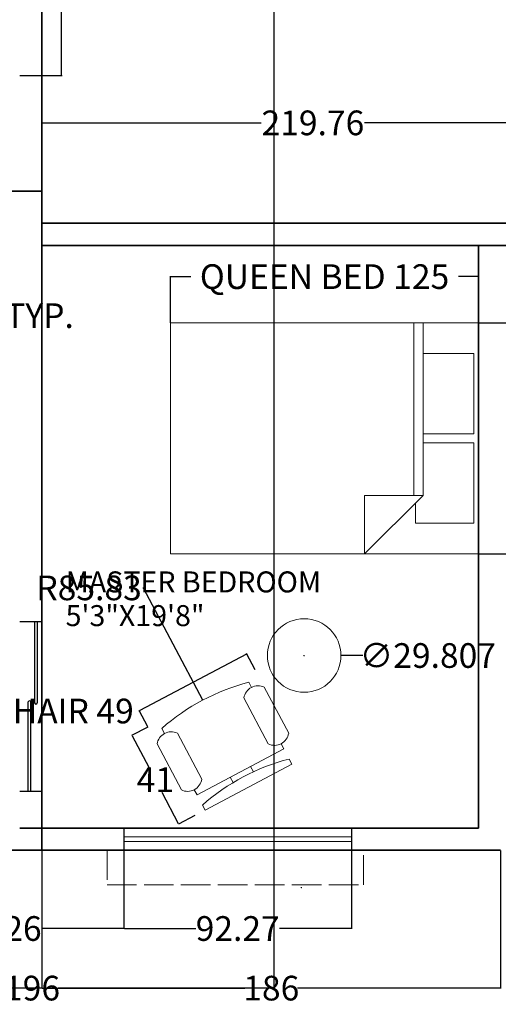
# Model space of a CAD drawing. Units: inches. Extents: x 135 to 880, y 60 to 879.
# Tile 2 of 5: x 363 to 557, y 60 to 459. Entities that reach past the tile are written whole.
import ezdxf

# ---------------------------------------------------------------- set-up
doc = ezdxf.new("R2010")
doc.units = ezdxf.units.IN
doc.header["$MEASUREMENT"] = 0
doc.linetypes.add('ACAD_ISO02W100', pattern=[15, 12, -3])
for name, color, linetype, lineweight in [('A-ANNO-DIMS', 2, 'Continuous', 18), ('A-AREA-IDEN', 7, 'Continuous', 18), ('A-DOOR', 3, 'Continuous', 25), ('A-FURN', 8, 'Continuous', 18), ('A-GLAZ', 4, 'Continuous', 18), ('A-ROOF-OVHD', 8, 'ACAD_ISO02W100', 18), ('A-WALL', 7, 'Continuous', 35)]:
    doc.layers.add(name, color=color, linetype=linetype, lineweight=lineweight)
doc.styles.get("Standard").update_dxf_attribs({"font": 'arial.ttf'})
doc.dimstyles.get("Standard").update_dxf_attribs({"dimtxt": 10, "dimasz": 0.18, "dimexe": 0.18, "dimexo": 0.0625, "dimgap": 0.09, "dimtad": 0, "dimtih": 1, "dimtoh": 1, "dimdec": 0, "dimzin": 0, "dimdsep": 46, "dimlunit": 3, "dimtxsty": 'Standard', "dimcen": 0.09, "dimadec": 0, "dimazin": 0, "dimtfac": 1, "dimtdec": 0, "dimtofl": 0, "dimtmove": 0, "dimatfit": 3, "dimfxl": 1, "dimtolj": 1, "dimtzin": 0, "dimarcsym": 0})

# ---------------------------------------------------------------- blocks, each defined once
blk = doc.blocks.new('Chair - Desk')
for p, q in [((-8.5, 0), (-8.5, -1)), ((-8.5, 0), (8.5, 0)), ((8.5, 0), (8.5, -1)), ((-8.5, -3), (-8.5, -4)), ((-8.5, -3), (8.5, -3)), ((-2, -3), (-2, -1.9355)), ((2, -1.9576), (2, -3)), ((8.5, -3), (8.5, -4)), ((-10.5, -5), (-10.5, -14)), ((-6.5, -14), (-6.5, -5)), ((6.5, -5), (6.5, -14)), ((10.5, -14), (10.5, -5)), ((-8.5, -15), (-8.5, -16)), ((8.5, -15), (8.5, -16))]:
    blk.add_line(p, q)
for centre, radius, start, end in [((0, 34.625), 36.625, 256.5803, 283.4197), ((-8.5, -6.5), 2.5, 36.8699, 143.1301), ((8.5, -6.5), 2.5, 36.8699, 143.1301), ((-8.5, -12.5), 2.5, 216.8699, 323.1301), ((8.5, -12.5), 2.5, 216.8699, 323.1301), ((0, 19.625), 36.625, 256.5803, 283.4197)]:
    blk.add_arc(centre, radius, start, end)
blk = doc.blocks.new('Bed - Queen')
for p, q in [((0, -80.00003), (0, 0)), ((0, 0), (59.99999, 0)), ((59.99999, 0), (59.99999, -80.00003)), ((7.99999, -1.2), (28.79998, -1.2)), ((7.99999, -14.4), (7.99999, -1.2)), ((28.79998, -1.2), (28.79998, -14.4)), ((31.19999, -1.2), (51.99999, -1.2)), ((31.19999, -14.4), (31.19999, -1.2)), ((51.99999, -1.2), (51.99999, -16.4)), ((0, -14.4), (44.8, -14.4)), ((59.99999, -29.6), (44.8, -14.4)), ((44.8, -14.4), (44.8, -29.6)), ((44.8, -16.8), (0, -16.8)), ((51.99999, -16.4), (46.79936, -16.4)), ((44.8, -29.6), (59.99999, -29.6)), ((59.99999, -80.00003), (0, -80.00003))]:
    blk.add_line(p, q)
blk = doc.blocks.new('*D14')
at = {"layer": 'A-ANNO-DIMS', "color": 0, "lineweight": -2, "transparency": 16777216}
for p, q in [((454.9, 202.13), (411.72, 179.27)), ((458.48, 195.75), (454.97, 202.38)), ((411.4, 179.11), (411.22, 179.11)), ((411.56, 179.19), (411.4, 179.11)), ((414.99, 172.72), (411.48, 179.35))]:
    blk.add_line(p, q, dxfattribs=at)
at = {"layer": 'A-ANNO-DIMS', "color": 0, "transparency": 16777216}
for points in [[(454.88, 202.16), (454.91, 202.11), (455.05, 202.22)], [(411.71, 179.3), (411.73, 179.25), (411.56, 179.19)]]:
    blk.add_solid(points, dxfattribs=at)
at = {"layer": 'Defpoints', "color": 0, "transparency": 16777216}
for p in [(458.51, 195.69), (411.56, 179.19), (415.01, 172.67)]:
    blk.add_point(p, dxfattribs=at)
at = {"layer": 'A-ANNO-DIMS', "color": 0, "transparency": 16777216, "insert": (380.34, 179.11), "char_height": 10, "attachment_point": 5}
blk.add_mtext('\\A1;CHAIR 49', dxfattribs=at)
blk = doc.blocks.new('*D15')
at = {"layer": 'A-ANNO-DIMS', "color": 0, "lineweight": -2, "transparency": 16777216}
for p, q in [((414.96, 172.64), (408.33, 169.13)), ((408.57, 169.05), (415.29, 156.37)), ((427.41, 133.47), (420.7, 146.15)), ((433.97, 136.74), (427.34, 133.23))]:
    blk.add_line(p, q, dxfattribs=at)
at = {"layer": 'A-ANNO-DIMS', "color": 0, "transparency": 16777216}
for points in [[(408.6, 169.07), (408.55, 169.04), (408.49, 169.21)], [(427.44, 133.48), (427.39, 133.46), (427.5, 133.31)]]:
    blk.add_solid(points, dxfattribs=at)
at = {"layer": 'Defpoints', "color": 0, "transparency": 16777216}
for p in [(415.01, 172.67), (434.02, 136.76), (427.5, 133.31)]:
    blk.add_point(p, dxfattribs=at)
at = {"layer": 'A-ANNO-DIMS', "color": 0, "transparency": 16777216, "insert": (417.99, 151.26), "char_height": 10, "attachment_point": 5}
blk.add_mtext('\\A1;41', dxfattribs=at)
blk = doc.blocks.new('*D25')
at = {"layer": 'A-ANNO-DIMS', "color": 0, "lineweight": -2, "transparency": 16777216}
for p, q in [((363.04, 521.66), (380.17, 521.66)), ((379.99, 521.48), (379.99, 484.31)), ((379.99, 436.75), (379.99, 473.92)), ((363.04, 436.57), (380.17, 436.57))]:
    blk.add_line(p, q, dxfattribs=at)
at = {"layer": 'A-ANNO-DIMS', "color": 0, "transparency": 16777216}
for points in [[(379.96, 521.48), (380.02, 521.48), (379.99, 521.66)], [(379.96, 436.75), (380.02, 436.75), (379.99, 436.57)]]:
    blk.add_solid(points, dxfattribs=at)
at = {"layer": 'Defpoints', "color": 0, "transparency": 16777216}
for p in [(362.98, 521.66), (362.98, 436.57), (379.99, 436.57)]:
    blk.add_point(p, dxfattribs=at)
at = {"layer": 'A-ANNO-DIMS', "color": 0, "transparency": 16777216, "insert": (379.99, 479.12), "char_height": 10, "attachment_point": 5}
blk.add_mtext('\\A1;85', dxfattribs=at)
blk = doc.blocks.new('*D26')
at = {"layer": 'A-ANNO-DIMS', "color": 0, "lineweight": -2, "transparency": 16777216}
for p, q in [((424.17, 336.45), (424.17, 355.29)), ((424.35, 355.11), (432.33, 355.11)), ((548.8, 355.11), (540.82, 355.11)), ((548.98, 336.45), (548.98, 355.29))]:
    blk.add_line(p, q, dxfattribs=at)
at = {"layer": 'A-ANNO-DIMS', "color": 0, "transparency": 16777216}
for points in [[(424.35, 355.14), (424.35, 355.08), (424.17, 355.11)], [(548.8, 355.14), (548.8, 355.08), (548.98, 355.11)]]:
    blk.add_solid(points, dxfattribs=at)
at = {"layer": 'Defpoints', "color": 0, "transparency": 16777216}
for p in [(548.98, 355.11), (424.17, 336.39), (548.98, 336.39)]:
    blk.add_point(p, dxfattribs=at)
at = {"layer": 'A-ANNO-DIMS', "color": 0, "transparency": 16777216, "insert": (486.57, 355.11), "char_height": 10, "attachment_point": 5}
blk.add_mtext('\\A1;QUEEN BED 125', dxfattribs=at)
blk = doc.blocks.new('*D27')
at = {"layer": 'A-ANNO-DIMS', "color": 0, "lineweight": -2, "transparency": 16777216}
for p, q in [((549.04, 336.39), (567.88, 336.39)), ((567.7, 336.21), (567.7, 294.78)), ((567.7, 242.96), (567.7, 284.39)), ((549.04, 242.78), (567.88, 242.78))]:
    blk.add_line(p, q, dxfattribs=at)
at = {"layer": 'A-ANNO-DIMS', "color": 0, "transparency": 16777216}
for points in [[(567.67, 336.21), (567.73, 336.21), (567.7, 336.39)], [(567.67, 242.96), (567.73, 242.96), (567.7, 242.78)]]:
    blk.add_solid(points, dxfattribs=at)
at = {"layer": 'Defpoints', "color": 0, "transparency": 16777216}
for p in [(548.98, 336.39), (548.98, 242.78), (567.7, 242.78)]:
    blk.add_point(p, dxfattribs=at)
at = {"layer": 'A-ANNO-DIMS', "color": 0, "transparency": 16777216, "insert": (567.7, 289.58), "char_height": 10, "attachment_point": 5}
blk.add_mtext('\\A1;94', dxfattribs=at)
blk = doc.blocks.new('*D32')
at = {"layer": 'A-ANNO-DIMS', "color": 0, "lineweight": -2, "transparency": 16777216}
for p, q in [((257.98, 344.64), (257.98, 339.12)), ((293.98, 344.64), (293.98, 339.12)), ((258.16, 339.3), (293.8, 339.3)), ((293.98, 339.3), (294.16, 339.3))]:
    blk.add_line(p, q, dxfattribs=at)
at = {"layer": 'A-ANNO-DIMS', "color": 0, "transparency": 16777216}
for points in [[(258.16, 339.33), (258.16, 339.27), (257.98, 339.3)], [(293.8, 339.33), (293.8, 339.27), (293.98, 339.3)]]:
    blk.add_solid(points, dxfattribs=at)
at = {"layer": 'Defpoints', "color": 0, "transparency": 16777216}
for p in [(257.98, 344.7), (293.98, 344.7), (293.98, 339.3)]:
    blk.add_point(p, dxfattribs=at)
at = {"layer": 'A-ANNO-DIMS', "color": 0, "transparency": 16777216, "insert": (341.23, 339.3), "char_height": 10, "attachment_point": 5}
blk.add_mtext('\\A1;DOOR 36 TYP.', dxfattribs=at)
blk = doc.blocks.new('*D54')
at = {"layer": 'A-ANNO-DIMS', "color": 0, "lineweight": -2, "transparency": 16777216}
for p, q in [((192.98, 122.64), (192.98, 66.67)), ((371.98, 122.64), (371.98, 66.67)), ((193.16, 66.85), (271.8, 66.85)), ((371.8, 66.85), (293.15, 66.85))]:
    blk.add_line(p, q, dxfattribs=at)
at = {"layer": 'A-ANNO-DIMS', "color": 0, "transparency": 16777216}
for points in [[(193.16, 66.88), (193.16, 66.82), (192.98, 66.85)], [(371.8, 66.88), (371.8, 66.82), (371.98, 66.85)]]:
    blk.add_solid(points, dxfattribs=at)
at = {"layer": 'Defpoints', "color": 0, "transparency": 16777216}
for p in [(192.98, 122.7), (371.98, 122.7), (371.98, 66.85)]:
    blk.add_point(p, dxfattribs=at)
at = {"layer": 'A-ANNO-DIMS', "color": 0, "transparency": 16777216, "insert": (282.48, 66.85), "char_height": 10, "attachment_point": 5}
blk.add_mtext('\\A1;179', dxfattribs=at)
blk = doc.blocks.new('*D55')
at = {"layer": 'A-ANNO-DIMS', "color": 0, "lineweight": -2, "transparency": 16777216}
for p, q in [((371.98, 122.64), (371.98, 66.67)), ((557.98, 122.64), (557.98, 66.67)), ((372.16, 66.85), (454.31, 66.85)), ((557.8, 66.85), (475.64, 66.85))]:
    blk.add_line(p, q, dxfattribs=at)
at = {"layer": 'A-ANNO-DIMS', "color": 0, "transparency": 16777216}
for points in [[(372.16, 66.88), (372.16, 66.82), (371.98, 66.85)], [(557.8, 66.88), (557.8, 66.82), (557.98, 66.85)]]:
    blk.add_solid(points, dxfattribs=at)
at = {"layer": 'Defpoints', "color": 0, "transparency": 16777216}
for p in [(371.98, 122.7), (557.98, 122.7), (557.98, 66.85)]:
    blk.add_point(p, dxfattribs=at)
at = {"layer": 'A-ANNO-DIMS', "color": 0, "transparency": 16777216, "insert": (464.98, 66.85), "char_height": 10, "attachment_point": 5}
blk.add_mtext('\\A1;186', dxfattribs=at)
blk = doc.blocks.new('*D59')
at = {"layer": 'A-ANNO-DIMS', "color": 0, "lineweight": -2, "transparency": 16777216}
for p, q in [((371.98, 131.64), (371.98, 90.82)), ((405.23, 131.64), (405.23, 90.82)), ((371.98, 91), (371.8, 91)), ((405.05, 91), (372.16, 91))]:
    blk.add_line(p, q, dxfattribs=at)
at = {"layer": 'A-ANNO-DIMS', "color": 0, "transparency": 16777216}
for points in [[(372.16, 91.03), (372.16, 90.97), (371.98, 91)], [(405.05, 91.03), (405.05, 90.97), (405.23, 91)]]:
    blk.add_solid(points, dxfattribs=at)
at = {"layer": 'Defpoints', "color": 0, "transparency": 16777216}
for p in [(371.98, 131.7), (405.23, 131.7), (371.98, 91)]:
    blk.add_point(p, dxfattribs=at)
at = {"layer": 'A-ANNO-DIMS', "color": 0, "transparency": 16777216, "insert": (354.84, 91), "char_height": 10, "attachment_point": 5}
blk.add_mtext('\\A1;33.26', dxfattribs=at)
blk = doc.blocks.new('*D60')
at = {"layer": 'A-ANNO-DIMS', "color": 0, "lineweight": -2, "transparency": 16777216}
for p, q in [((405.23, 131.64), (405.23, 90.82)), ((497.5, 131.64), (497.5, 90.82)), ((405.41, 91), (434.4, 91)), ((497.32, 91), (468.33, 91))]:
    blk.add_line(p, q, dxfattribs=at)
at = {"layer": 'A-ANNO-DIMS', "color": 0, "transparency": 16777216}
for points in [[(405.41, 91.03), (405.41, 90.97), (405.23, 91)], [(497.32, 91.03), (497.32, 90.97), (497.5, 91)]]:
    blk.add_solid(points, dxfattribs=at)
at = {"layer": 'Defpoints', "color": 0, "transparency": 16777216}
for p in [(405.23, 131.7), (497.5, 131.7), (405.23, 91)]:
    blk.add_point(p, dxfattribs=at)
at = {"layer": 'A-ANNO-DIMS', "color": 0, "transparency": 16777216, "insert": (451.37, 91), "char_height": 10, "attachment_point": 5}
blk.add_mtext('\\A1;92.27', dxfattribs=at)
blk = doc.blocks.new('*D72')
at = {"layer": 'A-ANNO-DIMS', "color": 0, "lineweight": -2, "transparency": 16777216}
for p, q in [((269.98, 822.64), (269.98, 66.67)), ((465.98, 822.64), (465.98, 66.67)), ((270.16, 66.85), (357.31, 66.85)), ((465.8, 66.85), (378.64, 66.85))]:
    blk.add_line(p, q, dxfattribs=at)
at = {"layer": 'A-ANNO-DIMS', "color": 0, "transparency": 16777216}
for points in [[(270.16, 66.88), (270.16, 66.82), (269.98, 66.85)], [(465.8, 66.88), (465.8, 66.82), (465.98, 66.85)]]:
    blk.add_solid(points, dxfattribs=at)
at = {"layer": 'Defpoints', "color": 0, "transparency": 16777216}
for p in [(269.98, 822.7), (465.98, 822.7), (465.98, 66.85)]:
    blk.add_point(p, dxfattribs=at)
at = {"layer": 'A-ANNO-DIMS', "color": 0, "transparency": 16777216, "insert": (367.98, 66.85), "char_height": 10, "attachment_point": 5}
blk.add_mtext('\\A1;196', dxfattribs=at)
blk = doc.blocks.new('*D74')
at = {"layer": 'A-ANNO-DIMS', "color": 0, "lineweight": -2, "transparency": 16777216}
for p, q in [((371.98, 376.76), (371.98, 417.58)), ((372.16, 417.4), (460.93, 417.4)), ((591.56, 417.4), (502.79, 417.4)), ((591.74, 376.76), (591.74, 417.58))]:
    blk.add_line(p, q, dxfattribs=at)
at = {"layer": 'A-ANNO-DIMS', "color": 0, "transparency": 16777216}
for points in [[(372.16, 417.43), (372.16, 417.37), (371.98, 417.4)], [(591.56, 417.43), (591.56, 417.37), (591.74, 417.4)]]:
    blk.add_solid(points, dxfattribs=at)
at = {"layer": 'Defpoints', "color": 0, "transparency": 16777216}
for p in [(591.74, 417.4), (371.98, 376.7), (591.74, 376.7)]:
    blk.add_point(p, dxfattribs=at)
at = {"layer": 'A-ANNO-DIMS', "color": 0, "transparency": 16777216, "insert": (481.86, 417.4), "char_height": 10, "attachment_point": 5}
blk.add_mtext('\\A1;219.76', dxfattribs=at)
blk = doc.blocks.new('*D80')
at = {"layer": 'A-ANNO-DIMS', "color": 0, "lineweight": -2, "transparency": 16777216}
for p, q in [((478.22, 201.6), (478.4, 201.6)), ((478.31, 201.51), (478.31, 201.69)), ((502.15, 201.6), (493.39, 201.6))]:
    blk.add_line(p, q, dxfattribs=at)
at = {"layer": 'A-ANNO-DIMS', "color": 0, "transparency": 16777216}
blk.add_solid([(493.39, 201.63), (493.39, 201.57), (493.21, 201.6)], dxfattribs=at)
at = {"layer": 'Defpoints', "color": 0, "transparency": 16777216}
for p in [(463.4, 201.6), (493.21, 201.6)]:
    blk.add_point(p, dxfattribs=at)
at = {"layer": 'A-ANNO-DIMS', "color": 0, "transparency": 16777216, "insert": (528.44, 201.6), "char_height": 10, "attachment_point": 5}
blk.add_mtext('\\A1;∅29.807', dxfattribs=at)
blk = doc.blocks.new('*D85')
at = {"layer": 'A-ANNO-DIMS', "color": 0, "lineweight": -2, "transparency": 16777216}
for p, q in [((412.85, 229), (413.03, 229)), ((413.03, 229), (437.04, 183.65)), ((477.29, 107.54), (477.29, 107.72)), ((477.2, 107.63), (477.38, 107.63))]:
    blk.add_line(p, q, dxfattribs=at)
at = {"layer": 'A-ANNO-DIMS', "color": 0, "transparency": 16777216}
blk.add_solid([(437.07, 183.66), (437.02, 183.63), (437.13, 183.49)], dxfattribs=at)
at = {"layer": 'Defpoints', "color": 0, "transparency": 16777216}
for p in [(437.13, 183.49), (477.29, 107.63)]:
    blk.add_point(p, dxfattribs=at)
at = {"layer": 'A-ANNO-DIMS', "color": 0, "transparency": 16777216, "insert": (391.1, 229), "char_height": 10, "attachment_point": 5}
blk.add_mtext('\\A1;R85.83', dxfattribs=at)

msp = doc.modelspace()

# ---------------------------------------------------------------- linework, layer by layer
at = {"layer": 'A-DOOR'}
for p, q in [((362.9753, 215.4206), (371.9753, 215.4206)), ((369.0511, 215.4206), (369.0511, 182.3912)), ((370.0511, 215.4206), (370.0511, 182.3912)), ((366.4743, 146.6389), (366.4743, 182.8082)), ((367.4743, 146.6389), (367.4743, 182.8082)), ((362.9753, 146.6389), (371.9753, 146.6389))]:
    msp.add_line(p, q, dxfattribs=at)
for centre, start, end in [((366.9743, 182.8082), 0, 180), ((369.5511, 182.3912), 180, 0)]:
    msp.add_arc(centre, 0.5, start, end, dxfattribs=at)
at = {"layer": 'A-FURN'}
msp.add_circle((478.3065, 201.5966), 14.9034, dxfattribs=at)
at = {"layer": 'A-GLAZ'}
for p, q in [((405.2334, 131.7014), (405.2334, 122.7014)), ((497.5015, 131.7014), (497.5015, 131.7014)), ((497.5015, 131.7014), (497.5015, 122.7014)), ((405.2334, 128.2014), (497.5015, 128.2014)), ((405.2334, 126.2014), (497.5015, 126.2014))]:
    msp.add_line(p, q, dxfattribs=at)
at = {"layer": 'A-ROOF-OVHD'}
for p, q in [((398.3792, 122.7014), (398.3792, 108.694)), ((502.332, 108.694), (502.332, 122.7014)), ((398.3792, 108.694), (502.332, 108.694))]:
    msp.add_line(p, q, dxfattribs=at)
at = {"layer": 'A-WALL'}
for p, q in [((371.9753, 559.7014), (371.9753, 389.7014)), ((371.9753, 389.7014), (343.1077, 389.7014)), ((371.9753, 258.7014), (371.9753, 389.7014)), ((775.9753, 376.7014), (371.9753, 376.7014)), ((784.9753, 367.7014), (371.9753, 367.7014)), ((548.9753, 131.7014), (548.9753, 367.7014)), ((548.9753, 367.7014), (557.9753, 367.7014)), ((371.9753, 122.7014), (371.9753, 258.7014)), ((362.9753, 131.7014), (371.9753, 131.7014)), ((371.9753, 131.7014), (548.9753, 131.7014)), ((192.9753, 122.7014), (371.9753, 122.7014)), ((371.9753, 122.7014), (557.9753, 122.7014))]:
    msp.add_line(p, q, dxfattribs=at)

# ---------------------------------------------------------------- block references
at = {"layer": 'A-FURN'}
for name, p, xscale, yscale, zscale, rotation in [('Bed - Queen', (548.9753, 336.3855), 1.560037282092657, 1.560037282092657, 1.560037282092657, 270), ('Chair - Desk', (455.7677, 148.2781), 2.343520009776944, 2.343520009776944, 2.343520009776944, 207.8972710309477)]:
    msp.add_blockref(name, p, dxfattribs=dict(at, xscale=xscale, yscale=yscale, zscale=zscale, rotation=rotation))

# ---------------------------------------------------------------- texts
at = {"layer": 'A-AREA-IDEN'}
for s, height, p in [('MASTER BEDROOM ', 8.505802, (381.5975, 227.1713)), ('5\'3"X19\'8"', 8.5058, (381.5975, 213.5075))]:
    msp.add_text(s, height=height, dxfattribs=at).set_placement(p)

# ---------------------------------------------------------------- dimensions: what is measured, and where the dimension line sits
at = {"layer": 'A-ANNO-DIMS'}
for base, p1, p2, override, picture, middle in [((465.9753, 66.853), (269.9753, 822.7014), (465.9753, 822.7014), {"dimdec": 0, "dimlfac": 1, "dimrnd": 0, "dimzin": 0, "dimdsep": 46, "dimlunit": 2}, '*D72', (367.9753, 66.853)), ((591.7388, 417.4014), (371.9753, 376.7014), (591.7388, 376.7014), {"dimdec": 2, "dimlfac": 1, "dimrnd": 0, "dimzin": 0, "dimdsep": 46, "dimlunit": 2}, '*D74', (481.8571, 417.4014)), ((371.9753, 66.853), (192.9753, 122.7014), (371.9753, 122.7014), {"dimdec": 0, "dimlfac": 1, "dimrnd": 0, "dimzin": 0, "dimdsep": 46, "dimlunit": 2}, '*D54', (282.4753, 66.853)), ((557.9753, 66.853), (371.9753, 122.7014), (557.9753, 122.7014), {"dimdec": 0, "dimlfac": 1, "dimrnd": 0, "dimzin": 0, "dimdsep": 46, "dimlunit": 2}, '*D55', (464.9753, 66.853))]:
    dim = msp.add_linear_dim(base=base, p1=p1, p2=p2, dimstyle='Standard', override=override, dxfattribs=at)
    dim.commit()
    dim.dimension.update_dxf_attribs({"geometry": picture, "text_midpoint": middle})
for base, p1, p2, angle, override, picture, middle in [((379.993, 436.5713), (362.9753, 521.6594), (362.9753, 436.5713), 270, {"dimdec": 0, "dimlfac": 1, "dimrnd": 0, "dimzin": 0, "dimdsep": 46, "dimlunit": 2}, '*D25', (379.993, 479.1154)), ((567.6958, 242.7833), (548.9753, 336.3855), (548.9753, 242.7833), 270, {"dimdec": 0, "dimlfac": 1, "dimrnd": 0, "dimzin": 0, "dimdsep": 46, "dimlunit": 2}, '*D27', (567.6958, 289.5844)), ((427.4961, 133.3108), (415.0143, 172.6652), (434.0203, 136.7648), 297.897271, {"dimdec": 0, "dimlfac": 1, "dimrnd": 0, "dimzin": 0, "dimdsep": 46, "dimlunit": 2}, '*D15', (417.9931, 151.261)), ((371.9753, 91.0014), (405.2334, 131.7014), (371.9753, 131.7014), 180, {"dimdec": 2, "dimlfac": 1, "dimrnd": 0, "dimzin": 0, "dimdsep": 46, "dimlunit": 2}, '*D59', (354.8397, 91.0014)), ((405.2334, 91.0014), (497.5015, 131.7014), (405.2334, 131.7014), 180, {"dimdec": 2, "dimlfac": 1, "dimrnd": 0, "dimzin": 0, "dimdsep": 46, "dimlunit": 2}, '*D60', (451.3674, 91.0014))]:
    dim = msp.add_linear_dim(base=base, p1=p1, p2=p2, angle=angle, dimstyle='Standard', override=override, dxfattribs=at)
    dim.commit()
    dim.dimension.update_dxf_attribs({"geometry": picture, "text_midpoint": middle})
for base, p1, p2, text, picture, middle in [((548.9753, 355.106), (424.1723, 336.3855), (548.9753, 336.3855), 'QUEEN BED <>', '*D26', (486.5738, 355.106)), ((293.9753, 339.3014), (257.9753, 344.7014), (293.9753, 344.7014), 'DOOR <> TYP.', '*D32', (341.2303, 339.3014))]:
    dim = msp.add_linear_dim(base=base, p1=p1, p2=p2, text=text, dimstyle='Standard', override={"dimdec": 0, "dimlfac": 1, "dimrnd": 0, "dimzin": 0, "dimdsep": 46, "dimlunit": 2}, dxfattribs=at)
    dim.commit()
    dim.dimension.update_dxf_attribs({"geometry": picture, "text_midpoint": middle})
dim = msp.add_radius_dim(center=(477.2866, 107.6313), mpoint=(437.127, 183.488), dimstyle='Standard', override={"dimdec": 2, "dimlfac": 1, "dimrnd": 0, "dimzin": 0, "dimdsep": 46, "dimlunit": 2}, dxfattribs=at)
dim.commit()
dim.dimension.update_dxf_attribs({"geometry": '*D85', "text_midpoint": (391.1037, 229.0021), "dimtype": 164})
dim = msp.add_diameter_dim_2p(p1=(463.4032, 201.5963), p2=(493.2099, 201.597), dimstyle='Standard', override={"dimdec": 3, "dimlfac": 1, "dimrnd": 0, "dimzin": 0, "dimdsep": 46, "dimlunit": 2}, dxfattribs=at)
dim.commit()
dim.dimension.update_dxf_attribs({"geometry": '*D80', "text_midpoint": (502.1519, 201.5972), "dimtype": 163})
dim = msp.add_linear_dim(base=(411.5603, 179.1894), p1=(458.5089, 195.6918), p2=(415.0143, 172.6652), angle=207.897271, text='CHAIR <>', dimstyle='Standard', override={"dimdec": 0, "dimlfac": 1, "dimrnd": 0, "dimzin": 0, "dimdsep": 46, "dimlunit": 2}, dxfattribs=at)
dim.commit()
dim.dimension.update_dxf_attribs({"geometry": '*D14', "text_midpoint": (380.3433, 179.1052)})

doc.saveas('drawing.dxf')
